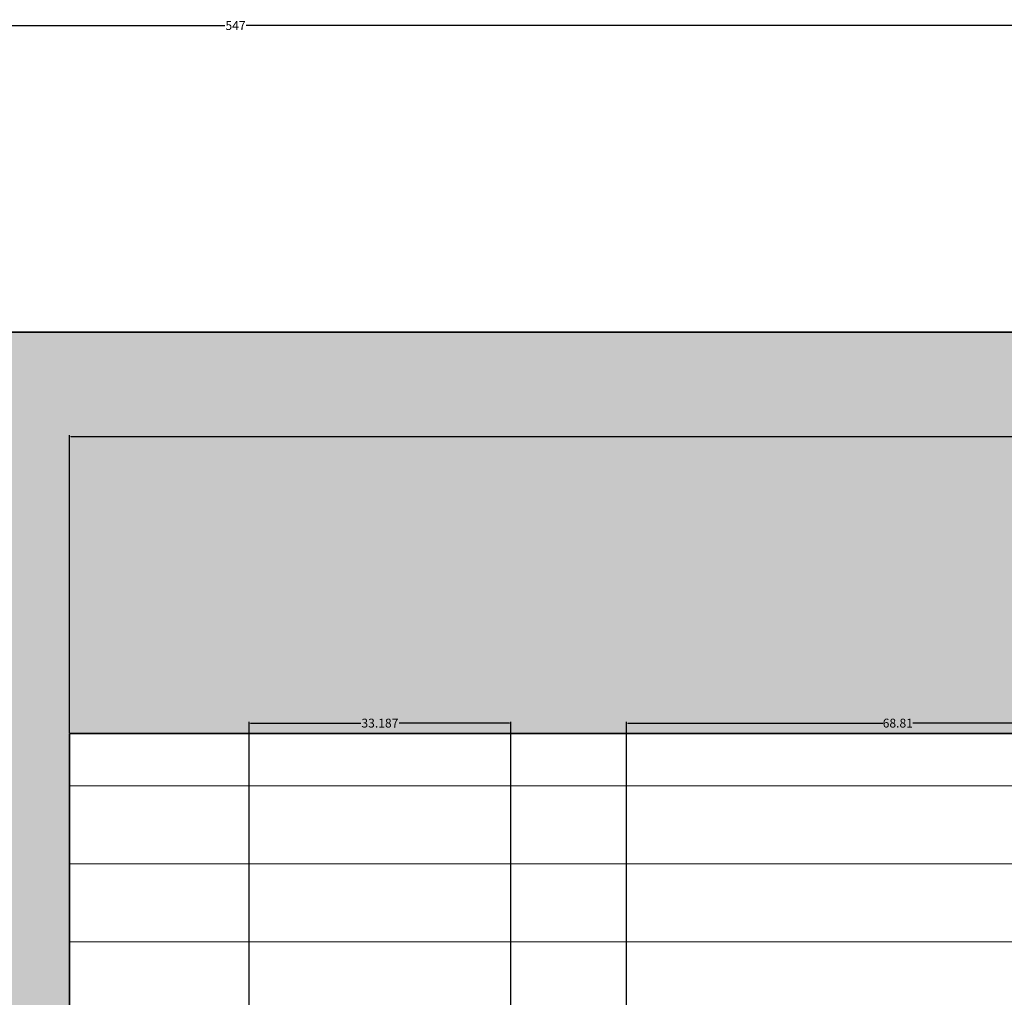
# Model space of a CAD drawing. Units: inches. Extents: x 8 to 634, y 41 to 867.
# Tile 19 of 21: x 293 to 418, y 743 to 867. Entities that reach past the tile are written whole.
import ezdxf

# ---------------------------------------------------------------- set-up
doc = ezdxf.new("R2010")
doc.units = ezdxf.units.IN
doc.header["$MEASUREMENT"] = 0
for name, color, linetype, lineweight in [('A-ANNO-DIMS', 2, 'Continuous', 18), ('A-ROOF', 7, 'Continuous', 35), ('A-ROOF-PATT', 8, 'Continuous', 9), ('A-WALL-PATT', 8, 'Continuous', 9)]:
    doc.layers.add(name, color=color, linetype=linetype, lineweight=lineweight)
doc.styles.get("Standard").update_dxf_attribs({"font": 'arial.ttf'})
doc.dimstyles.get("Standard").update_dxf_attribs({"dimtxt": 1.125, "dimasz": 0.18, "dimexe": 0.18, "dimexo": 0.0625, "dimgap": 0.09, "dimtad": 0, "dimtih": 1, "dimtoh": 1, "dimdec": 4, "dimzin": 0, "dimdsep": 46, "dimlunit": 4, "dimtxsty": 'Standard', "dimcen": 0.09, "dimadec": 0, "dimazin": 0, "dimtfac": 1, "dimtdec": 4, "dimtofl": 0, "dimtmove": 0, "dimatfit": 3, "dimfxl": 1, "dimtolj": 1, "dimtzin": 0, "dimarcsym": 0})

# ---------------------------------------------------------------- blocks, each defined once
blk = doc.blocks.new('*D19')
at = {"layer": 'A-ANNO-DIMS', "color": 0, "lineweight": -2, "transparency": 16777216}
for p, q in [((47.34, 697.73), (47.34, 866.81)), ((47.52, 866.63), (319.51, 866.63)), ((594.17, 866.63), (322.18, 866.63)), ((594.35, 827.83), (594.35, 866.81))]:
    blk.add_line(p, q, dxfattribs=at)
at = {"layer": 'A-ANNO-DIMS', "color": 0, "transparency": 16777216}
for points in [[(47.52, 866.66), (47.52, 866.6), (47.34, 866.63)], [(594.17, 866.66), (594.17, 866.6), (594.35, 866.63)]]:
    blk.add_solid(points, dxfattribs=at)
at = {"layer": 'Defpoints', "color": 0, "transparency": 16777216}
for p in [(594.35, 866.63), (594.35, 827.77), (47.34, 697.67)]:
    blk.add_point(p, dxfattribs=at)
at = {"layer": 'A-ANNO-DIMS', "color": 0, "transparency": 16777216, "insert": (320.85, 866.63), "char_height": 1.125, "attachment_point": 5}
blk.add_mtext('\\A1;547', dxfattribs=at)
blk = doc.blocks.new('*D47')
at = {"layer": 'A-ANNO-DIMS', "color": 0, "lineweight": -2, "transparency": 16777216}
for p, q in [((299.8, 776.96), (299.8, 814.72)), ((299.98, 814.54), (426.25, 814.54)), ((556.53, 814.54), (430.25, 814.54)), ((556.71, 776.96), (556.71, 814.72))]:
    blk.add_line(p, q, dxfattribs=at)
at = {"layer": 'A-ANNO-DIMS', "color": 0, "transparency": 16777216}
for points in [[(299.98, 814.57), (299.98, 814.51), (299.8, 814.54)], [(556.53, 814.57), (556.53, 814.51), (556.71, 814.54)]]:
    blk.add_solid(points, dxfattribs=at)
at = {"layer": 'Defpoints', "color": 0, "transparency": 16777216}
for p in [(556.71, 814.54), (299.8, 776.89), (556.71, 776.89)]:
    blk.add_point(p, dxfattribs=at)
at = {"layer": 'A-ANNO-DIMS', "color": 0, "transparency": 16777216, "insert": (428.25, 814.54), "char_height": 1.125, "attachment_point": 5}
blk.add_mtext('\\A1;256.9', dxfattribs=at)
blk = doc.blocks.new('*D48')
at = {"layer": 'A-ANNO-DIMS', "color": 0, "lineweight": -2, "transparency": 16777216}
for p, q in [((322.56, 740.62), (322.56, 778.39)), ((322.74, 778.21), (336.73, 778.21)), ((355.57, 778.21), (341.58, 778.21)), ((355.75, 740.62), (355.75, 778.39))]:
    blk.add_line(p, q, dxfattribs=at)
at = {"layer": 'A-ANNO-DIMS', "color": 0, "transparency": 16777216}
for points in [[(322.74, 778.24), (322.74, 778.18), (322.56, 778.21)], [(355.57, 778.24), (355.57, 778.18), (355.75, 778.21)]]:
    blk.add_solid(points, dxfattribs=at)
at = {"layer": 'Defpoints', "color": 0, "transparency": 16777216}
for p in [(355.75, 778.21), (322.56, 740.56), (355.75, 740.56)]:
    blk.add_point(p, dxfattribs=at)
at = {"layer": 'A-ANNO-DIMS', "color": 0, "transparency": 16777216, "insert": (339.15, 778.21), "char_height": 1.125, "attachment_point": 5}
blk.add_mtext('\\A1;33.187', dxfattribs=at)
blk = doc.blocks.new('*D50')
at = {"layer": 'A-ANNO-DIMS', "color": 0, "lineweight": -2, "transparency": 16777216}
for p, q in [((370.39, 740.62), (370.39, 778.39)), ((370.57, 778.21), (402.91, 778.21)), ((439.02, 778.21), (406.68, 778.21)), ((439.2, 740.62), (439.2, 778.39))]:
    blk.add_line(p, q, dxfattribs=at)
at = {"layer": 'A-ANNO-DIMS', "color": 0, "transparency": 16777216}
for points in [[(370.57, 778.24), (370.57, 778.18), (370.39, 778.21)], [(439.02, 778.24), (439.02, 778.18), (439.2, 778.21)]]:
    blk.add_solid(points, dxfattribs=at)
at = {"layer": 'Defpoints', "color": 0, "transparency": 16777216}
for p in [(439.2, 778.21), (370.39, 740.56), (439.2, 740.56)]:
    blk.add_point(p, dxfattribs=at)
at = {"layer": 'A-ANNO-DIMS', "color": 0, "transparency": 16777216, "insert": (404.79, 778.21), "char_height": 1.125, "attachment_point": 5}
blk.add_mtext('\\A1;68.81', dxfattribs=at)

msp = doc.modelspace()

# ---------------------------------------------------------------- hatches: boundary and pattern name
at = {"layer": 'A-ROOF-PATT', "transparency": 33554687}
h = msp.add_hatch(dxfattribs=at)
h.set_pattern_fill('AR-CONC', color=256, scale=2.2, angle=135)
h.paths.add_polyline_path([(262.2266, 828.9821), (144.3564, 828.9821), (144.3564, 697.6655), (262.2266, 785.231), (245.114, 785.231), (245.114, 792.8938), (262.2266, 792.8938)])
h.paths.add_polyline_path([(594.3501, 827.7671), (262.2266, 827.7671), (262.2266, 792.8938), (262.2266, 697.6655), (299.7961, 697.6655), (299.7961, 776.8929), (556.7072, 776.8929), (556.7072, 774.3342), (556.7072, 697.6655), (594.3501, 697.6655)])
at = {"layer": 'A-WALL-PATT', "transparency": 33554687}
h = msp.add_hatch(dxfattribs=at)
h.set_pattern_fill('ANSI31', color=256, scale=79, angle=135)
h.paths.add_polyline_path([(539.0002, 276.166), (499.4677, 276.166), (418.2881, 276.166), (418.2881, 228.4951), (435.5682, 228.4951), (539.0002, 228.4951)])
h.paths.add_polyline_path([(539.0002, 228.4951), (435.5682, 228.4951), (418.2881, 228.4951), (418.2881, 112.2342), (439.3242, 112.2342), (539.0002, 112.2342)])
h.paths.add_polyline_path([(518.1129, 124.2342), (473.3277, 124.2342), (473.3277, 216.4951), (518.1129, 216.4951)], flags=16)
h.paths.add_polyline_path([(451.2116, 124.2342), (427.4368, 124.2342), (427.4368, 216.4951), (451.2116, 216.4951)], flags=16)
h.paths.add_polyline_path([(539.0002, 112.2342), (439.3242, 112.2342), (418.2881, 112.2342), (418.2881, 91.5417), (539.0002, 91.5417)])
h.paths.add_polyline_path([(539.0002, 392.4268), (427.4368, 392.4268), (418.2881, 392.4268), (418.2881, 391.7598), (418.2881, 276.166), (499.4677, 276.166), (539.0002, 276.166)])
h.paths.add_polyline_path([(518.1129, 288.166), (473.3277, 288.166), (473.3277, 380.4268), (518.1129, 380.4268)], flags=16)
h.paths.add_polyline_path([(451.2116, 288.166), (427.4368, 288.166), (427.4368, 380.4268), (451.2116, 380.4268)], flags=16)
h.paths.add_polyline_path([(539.0002, 451.6305), (427.4368, 452.9097), (418.2881, 452.9097), (418.2881, 392.4268), (427.4368, 392.4268), (539.0002, 392.4268)])
h.paths.add_polyline_path([(539.0002, 569.1705), (427.4368, 569.1705), (418.2881, 569.1705), (418.2881, 452.9097), (427.4368, 452.9097), (539.0002, 451.6305)])
h.paths.add_polyline_path([(473.3277, 557.1705), (518.1129, 557.1705), (518.1129, 464.9097), (473.3277, 464.9097)], flags=16)
h.paths.add_polyline_path([(451.2116, 557.1705), (451.2116, 464.9097), (427.4368, 464.9097), (427.4368, 557.1705)], flags=16)
h.paths.add_polyline_path([(539.0002, 619.6298), (418.2881, 619.6298), (418.2881, 569.1705), (427.4368, 569.1705), (539.0002, 569.1705)])
h.paths.add_polyline_path([(556.7072, 774.3342), (556.7072, 776.8929), (299.7961, 776.8929), (299.7961, 697.6655), (322.56, 697.6655), (322.56, 740.5561), (355.7466, 740.5561), (355.7466, 697.6655), (360.785, 697.6655), (370.3877, 697.6655), (370.3877, 740.5561), (439.201, 740.5561), (439.201, 691.978), (449.4498, 691.978), (449.4498, 740.5561), (498.2535, 740.5561), (498.2535, 691.978), (508.5023, 691.978), (508.5023, 740.5561), (536.3204, 740.5561), (536.3204, 691.978), (539.0002, 691.978), (539.0002, 697.6655), (556.7072, 697.6655)])

# ---------------------------------------------------------------- linework, layer by layer
at = {"layer": 'A-ROOF'}
for p, q in [((594.3501, 827.7671), (262.2266, 827.7671)), ((299.7961, 697.6655), (299.7961, 776.8929)), ((299.7961, 776.8929), (556.7072, 776.8929))]:
    msp.add_line(p, q, dxfattribs=at)

# ---------------------------------------------------------------- dimensions: what is measured, and where the dimension line sits
at = {"layer": 'A-ANNO-DIMS'}
for base, p1, p2, override, picture, middle in [((594.3501, 866.6321), (47.3401, 697.6655), (594.3501, 827.7671), {"dimdec": 0, "dimlfac": 1, "dimrnd": 0, "dimzin": 0, "dimdsep": 46, "dimlunit": 2}, '*D19', (320.8451, 866.6321)), ((556.7072, 814.5429), (299.7961, 776.8929), (556.7072, 776.8929), {"dimdec": 1, "dimlfac": 1, "dimrnd": 0, "dimzin": 0, "dimdsep": 46, "dimlunit": 2}, '*D47', (428.2516, 814.5429)), ((355.7466, 778.2061), (322.56, 740.5561), (355.7466, 740.5561), {"dimdec": 3, "dimlfac": 1, "dimrnd": 0, "dimzin": 0, "dimdsep": 46, "dimlunit": 2}, '*D48', (339.1533, 778.2061)), ((439.201, 778.2061), (370.3877, 740.5561), (439.201, 740.5561), {"dimdec": 2, "dimlfac": 1, "dimrnd": 0, "dimzin": 0, "dimdsep": 46, "dimlunit": 2}, '*D50', (404.7943, 778.2061))]:
    dim = msp.add_linear_dim(base=base, p1=p1, p2=p2, dimstyle='Standard', override=override, dxfattribs=at)
    dim.commit()
    dim.dimension.update_dxf_attribs({"geometry": picture, "text_midpoint": middle})

doc.saveas('drawing.dxf')
